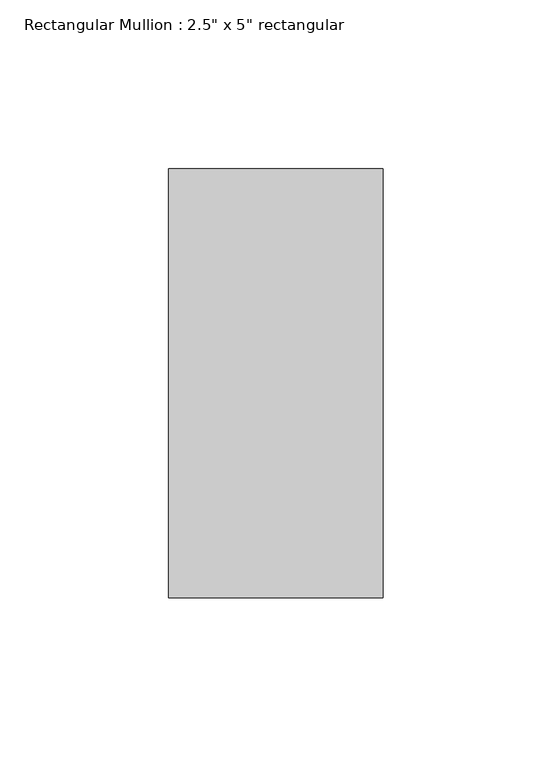
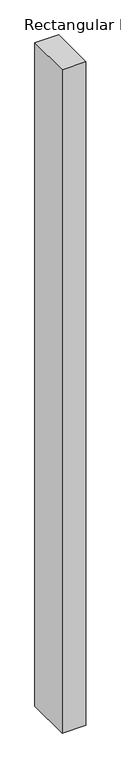
"""IFC4 building model written with IfcOpenShell, lengths in millimetres: member geometry."""

from ifc_helpers import new_model, si_unit, frame, origin, place, context, project, spatial, polyline, outline, extrude, source, transform, mapped, element, save


def member_33aca711(model_context):
    return source(origin(), model_context, "Body", "SweptSolid", [
        extrude(outline(polyline([(0.0, 63.5), (0.0, -63.5), (-63.5, -63.5), (-63.5, 63.5), (0.0, 63.5)])), frame((0.0, 0.0, -1885.7876892), z_axis=(0.0, 0.0, 1.0), x_axis=(1.0, 0.0, 0.0)), (0.0, 0.0, 1.0), 1885.7876892),
    ])


if __name__ == "__main__":
    model = new_model("IFC4")
    model_context = context("Model", 3, world=origin())
    ifc_project = project(units=[si_unit("LENGTHUNIT", "METRE", prefix="MILLI")], contexts=[model_context])
    site = spatial("IfcSite", under=ifc_project)
    building = spatial("IfcBuilding", under=site)
    placement = place(None, origin())
    member_shape = member_33aca711(model_context)
    element("IfcMember", 1, ObjectType="Rectangular Mullion : 2.5\" x 5\" rectangular", at=placement, inside=building, context=model_context, shape_type="MappedRepresentation", body=[
        mapped(member_shape, transform((0.0, 0.0, 0.0), x_axis=(1.0, 0.0, 0.0), y_axis=(0.0, 1.0, 0.0), z_axis=(0.0, 0.0, 1.0))),
    ])
    save(model, "model.ifc")

# Revit data of these elements
# Type "Rectangular Mullion : 2.5\" x 5\" rectangular"
#   built-in parameter 1007304 = 0.416667 (stored number, unit not read)
#   built-in parameter 1007301 = 0.104167 (stored number, unit not read)
#   built-in parameter 1007300 = 0.104167 (stored number, unit not read)
# Element 1 (IfcMember, "Rectangular Mullion : 2.5\" x 5\" rectangular")
#   Materials on its faces: "Aluminum"
# Materials
#   "Aluminum": class "Metal", colour RGB 247 247 247, transparency 0, Description = "Aluminum 6061", Cost = 0
